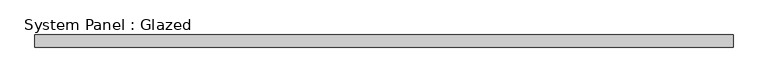
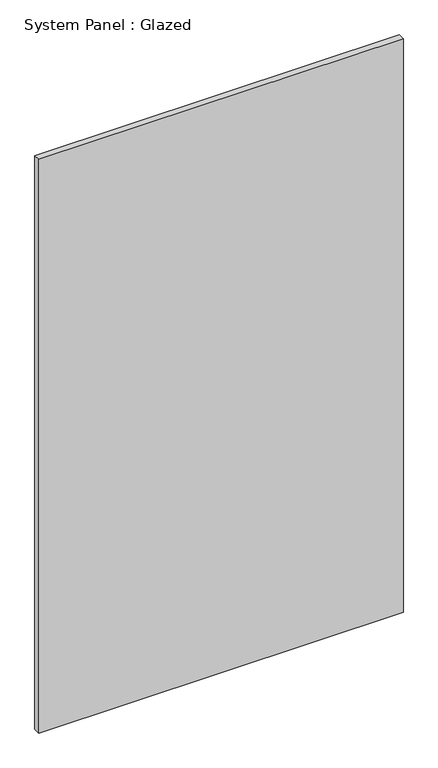
"""IFC4 building model written with IfcOpenShell, lengths in millimetres: plate geometry, System Panel : Glazed."""

from ifc_helpers import new_model, si_unit, origin, origin_with_axes, place, context, project, spatial, polyline, outline, extrude, source, transform, mapped, element, save


def system_panel_glazed_c89335d8(model_context):
    return source(origin(), model_context, "Body", "SweptSolid", [
        extrude(outline(polyline([(704.8499999, 19.05), (-704.8499999, 19.05), (-704.8499999, 44.45), (704.8499999, 44.45), (704.8499999, 19.05)])), origin_with_axes(), (0.0, 0.0, 1.0), 2343.15),
    ])


if __name__ == "__main__":
    model = new_model("IFC4")
    model_context = context("Model", 3, world=origin())
    ifc_project = project(units=[si_unit("LENGTHUNIT", "METRE", prefix="MILLI")], contexts=[model_context])
    site = spatial("IfcSite", under=ifc_project)
    building = spatial("IfcBuilding", under=site)
    placement = place(None, origin())
    system_panel_glazed_shape = system_panel_glazed_c89335d8(model_context)
    element("IfcPlate", 1, ObjectType="System Panel : Glazed", at=placement, inside=building, context=model_context, shape_type="MappedRepresentation", body=[
        mapped(system_panel_glazed_shape, transform((0.0, 0.0, 0.0), x_axis=(1.0, 0.0, 0.0), y_axis=(0.0, 1.0, 0.0), z_axis=(0.0, 0.0, 1.0))),
    ])
    save(model, "model.ifc")

# Revit data of these elements
# Type "System Panel : Glazed"
#   Construction Type Id = "GSP4R"
#   Analytic Construction = "1/8 in Pilkington single glazing"
#   Visual Light Transmittance = 0.9
#   Solar Heat Gain Coefficient = 0.86
#   Heat Transfer Coefficient (U) = 1.18115 BTU/(h·ft²·°F)
#   Define Thermal Properties by = 1
# Element 1 (IfcPlate, "System Panel : Glazed")
#   Materials on its faces: "Glass"
# Materials
#   "Glass": class "Glass", colour RGB 0 128 192, transparency 0.75, Description = "Soda Lime Glass", Cost = 0
